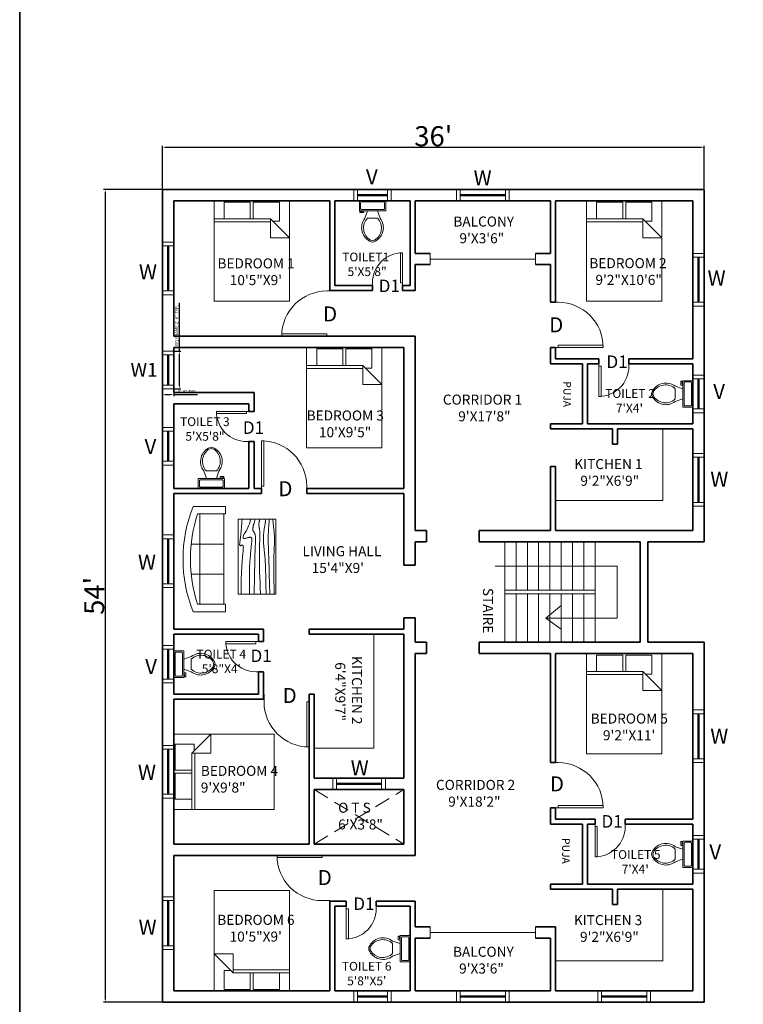
# Model space of a CAD drawing. Units: inches. Extents: x 2391 to 16591, y 7259 to 10239.
# Tile 17 of 27: x 2391 to 2968, y 8500 to 9285. Entities that reach past the tile are written whole.
import ezdxf

# ---------------------------------------------------------------- set-up
doc = ezdxf.new("R2010")
doc.units = ezdxf.units.IN
doc.linetypes.add('DASHED', pattern=[19.05, 12.7, -6.35])
for name, color, linetype, lineweight in [('A-ANNO-DIMS', 4, 'Continuous', 18), ('A-ANNO-IDEN', 2, 'Continuous', 18), ('A-ANNO-SYMB', 3, 'Continuous', 18), ('A-ANNO-TTLB', 7, 'Continuous', 35), ('A-AREA-IDEN', 7, 'Continuous', 18), ('A-DOOR', 3, 'Continuous', 18), ('A-FLOR-CASE', 6, 'Continuous', 18), ('A-FLOR-FIXT', 9, 'Continuous', 18), ('A-FLOR-HRAL', 8, 'Continuous', 18), ('A-FLOR-OPEN', 4, 'DASHED', 13), ('A-FLOR-STRS', 7, 'Continuous', 18), ('A-FURN', 8, 'Continuous', 18), ('A-GLAZ', 4, 'Continuous', 18), ('A-WALL', 7, 'Continuous', 35)]:
    doc.layers.add(name, color=color, linetype=linetype, lineweight=lineweight)
doc.styles.get("Standard").update_dxf_attribs({"font": 'arial.ttf'})
doc.dimstyles.new('ISO-25', dxfattribs={"dimtxt": 2.5, "dimasz": 2.5, "dimexe": 1.25, "dimexo": 0.625, "dimtad": 1, "dimdec": 0, "dimlunit": 3, "dimtxsty": 'Standard', "dimcen": 2.5, "dimadec": 0, "dimazin": 0, "dimtfac": 1, "dimtdec": 0, "dimtmove": 0, "dimatfit": 3, "dimfxl": 1, "dimarcsym": 0})

# ---------------------------------------------------------------- blocks, each defined once
blk = doc.blocks.new('Bed - Queen')
for p, q in [((0, -80.00003), (0, 0)), ((0, 0), (59.99999, 0)), ((59.99999, 0), (59.99999, -80.00003)), ((7.99999, -1.2), (28.79998, -1.2)), ((7.99999, -14.4), (7.99999, -1.2)), ((28.79998, -1.2), (28.79998, -14.4)), ((31.19999, -1.2), (51.99999, -1.2)), ((31.19999, -14.4), (31.19999, -1.2)), ((51.99999, -1.2), (51.99999, -16.4)), ((0, -14.4), (44.8, -14.4)), ((59.99999, -29.6), (44.8, -14.4)), ((44.8, -14.4), (44.8, -29.6)), ((44.8, -16.8), (0, -16.8)), ((51.99999, -16.4), (46.79936, -16.4)), ((44.8, -29.6), (59.99999, -29.6)), ((59.99999, -80.00003), (0, -80.00003))]:
    blk.add_line(p, q)
blk = doc.blocks.new('Toilet - top')
for p, q in [((9.5, -6), (9.5, -2)), ((-10, -8.5), (-8, -8.5)), ((-10, -9.5), (-10, -8.5)), ((-7, -9.5), (-10, -9.5)), ((-8, -8.5), (-8, -8)), ((-7, -8), (-7, -9.5)), ((-4, -8), (-6, -14)), ((4, -14), (-4, -14)), ((4, -8), (6, -14))]:
    blk.add_line(p, q)
blk.add_lwpolyline([(10.5, -8), (10.5, 0), (-10.5, 0), (-10.5, -8)], close=True)
for points in [[(-9.5, -2), (-9.5, -6)], [(8.5, -1), (-8.5, -1)], [(-8.5, -7), (8.5, -7)]]:
    blk.add_lwpolyline(points)
for centre, radius, start, end in [((-8.62, -1.88), 0.884, 81.8699, 188.1301), ((-8.62, -6.12), 0.884, 171.8699, 278.1301), ((8.62, -1.88), 0.884, 351.8699, 98.1301), ((8.62, -6.12), 0.884, 261.8699, 8.1301), ((3.52, -21.58), 12.17, 141.46911, 247.97143), ((4.2, -21.82), 11.33, 136.36773, 238.94682), ((-3.52, -21.58), 12.17, 292.02843, 38.53071), ((-4.2, -21.82), 11.33, 301.05301, 43.63209), ((0, -27.88), 4, 245.73182, 294.26817), ((0, -29), 4, 254.86053, 285.13947)]:
    blk.add_arc(centre, radius, start, end)
blk = doc.blocks.new('Sofa - Roundback 7 ft.')
for p, q in [((-12.00002, -32.4421), (-12.00003, -6.5971)), ((11.99997, -32.4421), (11.99998, -6.5971)), ((-36.000027, -34), (-36.000027, -11.4696)), ((-35.999844, -13.3819), (35.9998, -13.3819)), ((35.99998, -34), (35.99998, -11.4696)), ((-36.000027, -32.4421), (35.99998, -32.4421))]:
    blk.add_line(p, q)
for points in [[(-36.000027, -34), (-42.000027, -34), (-42.000027, -8)], [(41.99998, -8), (41.99998, -34), (35.99998, -34)]]:
    blk.add_lwpolyline(points)
for centre, radius, start, end in [((0, -114.25), 114.25, 68.43141, 111.5686), ((-0.00001, -127.1968), 121.1968, 72.72033, 107.2797)]:
    blk.add_arc(centre, radius, start, end)
blk = doc.blocks.new('Table - Rectangular Woodgrain 60 x 30 in.')
for p, q in [((0, 0), (0, -30)), ((60, 0), (0, 0)), ((60, -30), (60, 0)), ((0, -30), (60, -30))]:
    blk.add_line(p, q)
for points in [[(0, -2.4), (4.8155, -2.418), (9.0302, -2.4688), (12.709, -2.5477), (15.9167, -2.65), (18.7181, -2.7711), (21.1781, -2.9063), (23.3616, -3.0508), (25.3333, -3.2), (27.1477, -3.3495), (28.8172, -3.4958), (30.3437, -3.636), (31.7291, -3.7667), (32.9756, -3.8849), (34.0849, -3.9875), (35.059, -4.0714), (35.9, -4.1334), (36.6114, -4.1711), (37.2041, -4.1854), (37.6906, -4.1779), (38.0833, -4.15), (38.3948, -4.1034), (38.6375, -4.0396), (38.8239, -3.9602), (38.9666, -3.8667), (39.0764, -3.7608), (39.1573, -3.6448), (39.2116, -3.521), (39.2416, -3.3917), (39.2498, -3.2593), (39.2385, -3.1261), (39.21, -2.9944), (39.1666, -2.8667), (39.111, -2.7447), (39.0468, -2.6281), (38.978, -2.5163), (38.9083, -2.4083), (38.8418, -2.3035), (38.7823, -2.201), (38.7337, -2.1001), (38.7, -2), (38.6844, -1.9003), (38.6875, -1.8021), (38.7094, -1.707), (38.75, -1.6167), (38.8094, -1.5326), (38.8875, -1.4563), (38.9844, -1.3893), (39.1, -1.3333), (39.2351, -1.2896), (39.3937, -1.2583), (39.5804, -1.2396), (39.8, -1.2333), (40.057, -1.2396), (40.3562, -1.2583), (40.7023, -1.2896), (41.1, -1.3333), (41.5547, -1.3895), (42.0755, -1.4573), (42.6721, -1.5361), (43.3542, -1.625), (44.1316, -1.7233), (45.014, -1.8302), (46.0114, -1.9449), (47.1333, -2.0667), (48.3862, -2.1947), (49.7625, -2.3281), (51.2513, -2.4663), (52.8416, -2.6083), (54.5226, -2.7535), (56.2833, -2.9011), (58.1127, -3.0501), (60, -3.2)], [(0, -9.2), (6.5759, -9.0858), (11.9385, -9.0365), (16.2527, -9.0418), (19.6833, -9.0917), (22.3952, -9.1759), (24.5531, -9.2844), (26.322, -9.4069), (27.8666, -9.5333), (29.3241, -9.6553), (30.7203, -9.7719), (32.0532, -9.8837), (33.3208, -9.9917), (34.5213, -10.0965), (35.6526, -10.199), (36.7128, -10.2999), (37.7, -10.4), (38.6129, -10.4996), (39.4531, -10.5969), (40.223, -10.6895), (40.925, -10.775), (41.5613, -10.8512), (42.1344, -10.9156), (42.6465, -10.966), (43.1, -11), (43.4976, -11.0158), (43.8437, -11.0136), (44.143, -10.9942), (44.4, -10.9583), (44.6195, -10.9069), (44.8062, -10.8406), (44.9648, -10.7603), (45.1, -10.6667), (45.2155, -10.5598), (45.3114, -10.4365), (45.3871, -10.2929), (45.4416, -10.125), (45.4743, -9.929), (45.4844, -9.7011), (45.4709, -9.4371), (45.4333, -9.1333), (45.3716, -8.7883), (45.2896, -8.4104), (45.1919, -8.0107), (45.0833, -7.6), (44.9685, -7.1893), (44.8521, -6.7896), (44.7388, -6.4117), (44.6333, -6.0667), (44.54, -5.7628), (44.4614, -5.4979), (44.4001, -5.2675), (44.3583, -5.0667), (44.3384, -4.8909), (44.3427, -4.7354), (44.3736, -4.5956), (44.4333, -4.4667), (44.5236, -4.3453), (44.6427, -4.2333), (44.7884, -4.1339), (44.9583, -4.05), (45.1501, -3.9849), (45.3614, -3.9417), (45.59, -3.9234), (45.8333, -3.9333), (46.0915, -3.9749), (46.3734, -4.0531), (46.6906, -4.1736), (47.0542, -4.3417), (47.4756, -4.5629), (47.9661, -4.8427), (48.5372, -5.1866), (49.2, -5.6), (49.9676, -6.0844), (50.8594, -6.625), (51.8965, -7.2031), (53.1, -7.8), (54.491, -8.3969), (56.0906, -8.975), (57.9199, -9.5156), (60, -10)], [(0, -12.8), (5.1847, -12.9322), (9.6213, -13.0323), (13.3963, -13.1059), (16.5958, -13.1583), (19.3063, -13.1952), (21.614, -13.2219), (23.6054, -13.2439), (25.3666, -13.2667), (26.9728, -13.2947), (28.4531, -13.3281), (29.8256, -13.3663), (31.1083, -13.4083), (32.3191, -13.4535), (33.476, -13.501), (34.597, -13.5501), (35.7, -13.6), (36.7984, -13.6497), (37.8875, -13.6979), (38.9578, -13.743), (40, -13.7833), (41.0047, -13.8174), (41.9625, -13.8438), (42.864, -13.8607), (43.7, -13.8667), (44.4631, -13.8604), (45.1552, -13.8417), (45.7801, -13.8104), (46.3416, -13.7667), (46.8439, -13.7104), (47.2906, -13.6417), (47.6858, -13.5604), (48.0333, -13.4667), (48.3375, -13.3608), (48.6042, -13.2448), (48.8396, -13.121), (49.05, -12.9917), (49.2417, -12.8593), (49.4208, -12.7261), (49.5937, -12.5944), (49.7667, -12.4667), (49.9452, -12.3451), (50.1323, -12.2313), (50.3303, -12.1268), (50.5416, -12.0333), (50.7686, -11.9524), (51.0135, -11.8854), (51.2788, -11.8341), (51.5666, -11.8), (51.8785, -11.7843), (52.2116, -11.7865), (52.562, -11.8059), (52.926, -11.8417), (53.2998, -11.8931), (53.6795, -11.9594), (54.0614, -12.0397), (54.4416, -12.1333), (54.8223, -12.2401), (55.2293, -12.3625), (55.6942, -12.5037), (56.2489, -12.6667), (56.9251, -12.8547), (57.7545, -13.0708), (58.7689, -13.3182), (60, -13.6)], [(0, -18), (5.124, -17.7273), (9.6609, -17.5057), (13.6705, -17.3303), (17.2125, -17.1958), (20.3467, -17.0973), (23.1328, -17.0297), (25.6307, -16.9878), (27.9, -16.9667), (29.9928, -16.9617), (31.9302, -16.9703), (33.7254, -16.9907), (35.3917, -17.0208), (36.9423, -17.0588), (38.3906, -17.1026), (39.7499, -17.1503), (41.0333, -17.2), (42.2519, -17.2496), (43.4073, -17.2969), (44.4986, -17.3395), (45.525, -17.375), (46.4858, -17.4012), (47.3802, -17.4156), (48.2074, -17.416), (48.9667, -17.4), (49.6583, -17.3662), (50.2872, -17.3167), (50.8595, -17.2547), (51.3812, -17.1833), (51.8584, -17.1057), (52.2971, -17.025), (52.7034, -16.9443), (53.0833, -16.8667), (53.443, -16.7951), (53.789, -16.7313), (54.128, -16.6768), (54.4666, -16.6334), (54.8115, -16.6024), (55.1693, -16.5854), (55.5465, -16.5841), (55.95, -16.6), (56.3828, -16.6337), (56.8346, -16.6823), (57.2915, -16.7418), (57.7396, -16.8084), (58.165, -16.878), (58.5539, -16.9469), (58.8924, -17.0111), (59.1666, -17.0667), (59.3679, -17.1107), (59.5078, -17.1438), (59.6032, -17.1675), (59.6708, -17.1833), (59.7275, -17.193), (59.7901, -17.1979), (59.8753, -17.1998), (60, -17.2)], [(0, -22.4), (8.0098, -22.2501), (14.4094, -22.1011), (19.4168, -21.9535), (23.25, -21.8083), (26.1269, -21.6663), (28.2656, -21.5281), (29.884, -21.3947), (31.2, -21.2667), (32.3967, -21.1448), (33.5172, -21.0292), (34.5697, -20.9198), (35.5625, -20.8167), (36.5037, -20.7198), (37.4015, -20.6292), (38.2642, -20.5448), (39.1, -20.4667), (39.9164, -20.3951), (40.7187, -20.3313), (41.5117, -20.2768), (42.3, -20.2333), (43.0883, -20.2024), (43.8812, -20.1854), (44.6836, -20.1841), (45.5, -20.2), (46.3328, -20.234), (47.1747, -20.2844), (48.0163, -20.3488), (48.8479, -20.425), (49.66, -20.5106), (50.4429, -20.6031), (51.1872, -20.7004), (51.8833, -20.8), (52.5246, -20.8999), (53.1166, -20.9995), (53.6681, -21.0983), (54.1875, -21.1958), (54.6834, -21.2919), (55.1646, -21.3859), (55.6394, -21.4777), (56.1167, -21.5667), (56.6028, -21.6515), (57.0961, -21.7266), (57.5929, -21.7852), (58.0896, -21.8208), (58.5823, -21.8268), (59.0674, -21.7964), (59.5412, -21.723), (60, -21.6)], [(0, -25.2), (8.6355, -25.0504), (15.7026, -24.9031), (21.4049, -24.7606), (25.9458, -24.625), (29.529, -24.4988), (32.3578, -24.3844), (34.6359, -24.284), (36.5667, -24.2), (38.3213, -24.1341), (39.9417, -24.0854), (41.437, -24.0523), (42.8167, -24.0333), (44.0901, -24.0268), (45.2667, -24.0313), (46.3557, -24.0451), (47.3667, -24.0667), (48.309, -24.0947), (49.1928, -24.1287), (50.0284, -24.168), (50.826, -24.2125), (51.5959, -24.2617), (52.3483, -24.3151), (53.0935, -24.3725), (53.8417, -24.4334), (54.6009, -24.497), (55.3699, -24.561), (56.1454, -24.6226), (56.9239, -24.6792), (57.7021, -24.7279), (58.4764, -24.7662), (59.2435, -24.7911), (60, -24.8)], [(0, -28.8), (5.6867, -28.6681), (10.45, -28.5698), (14.407, -28.5012), (17.675, -28.4584), (20.3711, -28.4374), (22.6125, -28.4344), (24.5164, -28.4455), (26.2, -28.4667), (27.762, -28.4947), (29.2276, -28.5281), (30.6033, -28.5663), (31.8958, -28.6084), (33.1118, -28.6535), (34.2578, -28.7011), (35.3405, -28.7501), (36.3666, -28.8), (37.3443, -28.8497), (38.288, -28.8974), (39.2137, -28.9412), (40.1375, -28.9792), (41.0753, -29.0093), (42.0432, -29.0297), (43.0572, -29.0384), (44.1333, -29.0333), (45.2936, -29.0114), (46.5843, -28.9641), (48.0579, -28.8816), (49.7666, -28.7542), (51.7629, -28.5721), (54.0989, -28.3255), (56.8272, -28.0048), (60, -27.6)]]:
    blk.add_lwpolyline(points)
blk = doc.blocks.new('*U7')
for p, q in [((0, 0), (0, -6)), ((36, 0), (36, -6))]:
    blk.add_line(p, q)
blk.add_lwpolyline([(0, 0), (0, 36), (1.75, 36), (1.75, 0)], close=True)
blk.add_arc((0, 0), 36, 0, 90)
blk = doc.blocks.new('*U6')
for p, q in [((-36, 0), (-36, 6)), ((0, 0), (0, 6))]:
    blk.add_line(p, q)
blk.add_lwpolyline([(0, 0), (0, -36), (-1.75, -36), (-1.75, 0)], close=True)
blk.add_arc((0, 0), 36, 180, 270)
blk = doc.blocks.new('*U8')
for p, q in [((-24, 0), (-24, -6)), ((0, 0), (0, -6))]:
    blk.add_line(p, q)
blk.add_lwpolyline([(0, 0), (0, 24), (-1.75, 24), (-1.75, 0)], close=True)
blk.add_arc((0, 0), 24, 90, 180)
blk = doc.blocks.new('*U9')
for p, q in [((0, 0), (0, 6)), ((24, 0), (24, 6))]:
    blk.add_line(p, q)
blk.add_lwpolyline([(0, 0), (0, -24), (1.75, -24), (1.75, 0)], close=True)
blk.add_arc((0, 0), 24, 270, 0)
blk = doc.blocks.new('*U10')
for p, q in [((0, 0), (0, -6)), ((-36, 0), (-36, -6))]:
    blk.add_line(p, q)
blk.add_lwpolyline([(0, 0), (0, 36), (-1.75, 36), (-1.75, 0)], close=True)
blk.add_arc((0, 0), 36, 90, 180)
blk = doc.blocks.new('*U11')
for p, q in [((-36, 0), (-36, 6)), ((0, 0), (0, 6))]:
    blk.add_line(p, q)
blk.add_lwpolyline([(0, 0), (0, -36), (-1.75, -36), (-1.75, 0)], close=True)
blk.add_arc((0, 0), 36, 180, 270)
blk = doc.blocks.new('*U12')
for p, q in [((0, 0), (0, -6)), ((-36, 0), (-36, -6))]:
    blk.add_line(p, q)
blk.add_lwpolyline([(0, 0), (0, 36), (-1.75, 36), (-1.75, 0)], close=True)
blk.add_arc((0, 0), 36, 90, 180)
blk = doc.blocks.new('*U13')
for p, q in [((0, 0), (0, 6)), ((36, 0), (36, 6))]:
    blk.add_line(p, q)
blk.add_lwpolyline([(0, 0), (0, -36), (1.75, -36), (1.75, 0)], close=True)
blk.add_arc((0, 0), 36, 270, 0)
blk = doc.blocks.new('*D14')
at = {"layer": 'A-ANNO-DIMS', "color": 0, "lineweight": -2, "transparency": 16777216}
for p, q in [((2505.16, 9150.16), (2505.16, 9184.36)), ((2937.16, 9150.16), (2937.16, 9184.36)), ((2507.66, 9183.11), (2934.66, 9183.11))]:
    blk.add_line(p, q, dxfattribs=at)
at = {"layer": 'A-ANNO-DIMS', "color": 0, "transparency": 16777216}
for points in [[(2507.66, 9183.53), (2507.66, 9182.7), (2505.16, 9183.11)], [(2934.66, 9183.53), (2934.66, 9182.7), (2937.16, 9183.11)]]:
    blk.add_solid(points, dxfattribs=at)
at = {"layer": 'Defpoints', "color": 0, "transparency": 16777216}
for p in [(2937.16, 9183.11), (2505.16, 9149.53), (2937.16, 9149.53)]:
    blk.add_point(p, dxfattribs=at)
at = {"layer": 'A-ANNO-DIMS', "color": 0, "transparency": 16777216, "insert": (2721.16, 9191.91), "char_height": 2.5, "attachment_point": 5}
blk.add_mtext("{\\H6.4x;36'}", dxfattribs=at)
blk = doc.blocks.new('*D15')
at = {"layer": 'A-ANNO-DIMS', "color": 0, "lineweight": -2, "transparency": 16777216}
for p, q in [((2504.54, 9149.53), (2458.23, 9149.53)), ((2459.48, 9147.03), (2459.48, 8504.03)), ((2504.54, 8501.53), (2458.23, 8501.53))]:
    blk.add_line(p, q, dxfattribs=at)
at = {"layer": 'A-ANNO-DIMS', "color": 0, "transparency": 16777216}
for points in [[(2459.06, 9147.03), (2459.89, 9147.03), (2459.48, 9149.53)], [(2459.06, 8504.03), (2459.89, 8504.03), (2459.48, 8501.53)]]:
    blk.add_solid(points, dxfattribs=at)
at = {"layer": 'Defpoints', "color": 0, "transparency": 16777216}
for p in [(2505.16, 9149.53), (2459.48, 8501.53), (2505.16, 8501.53)]:
    blk.add_point(p, dxfattribs=at)
at = {"layer": 'A-ANNO-DIMS', "color": 0, "transparency": 16777216, "insert": (2450.71, 8825.53), "char_height": 2.5, "attachment_point": 5, "rotation": 90}
blk.add_mtext("{\\H6.4x;54'}", dxfattribs=at)
blk = doc.blocks.new('WINDOW-36-PLAN')
for p, q in [((9, 42), (0, 42)), ((9, 39), (0, 39)), ((4, 39), (4, 3)), ((4.5, 39), (4.5, 3)), ((5, 39), (5, 3)), ((9, 3), (0, 3)), ((9, 0), (0, 0))]:
    blk.add_line(p, q)
blk = doc.blocks.new('VENT-24-PLAN')
for p, q in [((9, 30), (0, 30)), ((9, 27), (0, 27)), ((4, 27), (4, 3)), ((4.5, 27), (4.5, 3)), ((5, 27), (5, 3)), ((9, 3), (0, 3)), ((9, 0), (0, 0))]:
    blk.add_line(p, q)
blk = doc.blocks.new('WINDOW-24-PLAN')
for p, q in [((9, 30), (0, 30)), ((9, 27), (0, 27)), ((4, 27), (4, 3)), ((4.5, 27), (4.5, 3)), ((5, 27), (5, 3)), ((9, 3), (0, 3)), ((9, 0), (0, 0))]:
    blk.add_line(p, q)
blk = doc.blocks.new('STAIR-RETURN-FLIGHT')
for p, q in [((0, 80), (0, 0)), ((9, 80), (9, 41.5)), ((18, 80), (18, 41.5)), ((27, 80), (27, 41.5)), ((36, 80), (36, 41.5)), ((45, 80), (45, 41.5)), ((54, 80), (54, 41.5)), ((63, 80), (63, 41.5)), ((72, 80), (72, 0)), ((72, 41.5), (0, 41.5)), ((72, 38.5), (0, 38.5)), ((9, 38.5), (9, 0)), ((18, 38.5), (18, 0)), ((27, 38.5), (27, 0)), ((36, 38.5), (36, 0)), ((45, 38.5), (45, 0)), ((54, 38.5), (54, 0)), ((63, 38.5), (63, 0))]:
    blk.add_line(p, q)
blk = doc.blocks.new('STAIR-DIRECTION-ARROW')
for p, q in [((0, 50.31), (97.37, 50.31)), ((97.37, 50.31), (97.37, 8.81)), ((40.34, 8.81), (52.74, 18.89)), ((97.37, 8.81), (40.34, 8.81)), ((40.34, 8.81), (52.74, 0))]:
    blk.add_line(p, q)
blk = doc.blocks.new('COUNTER-L-RETURN')
for q in [(47.5, 91), (0, 0)]:
    blk.add_line((47.5, 0), q)
blk = doc.blocks.new('COUNTER-L-KITCHEN')
for p, q in [((85.5, 57), (85.5, 0)), ((85.5, 0), (0, 0))]:
    blk.add_line(p, q)
blk = doc.blocks.new('*D41')
at = {"layer": 'A-ANNO-DIMS', "color": 0, "lineweight": -2, "transparency": 16777216}
for p, q in [((2518.66, 9020.53), (2518.66, 9059.02)), ((2514.79, 9020.53), (2519.91, 9020.53)), ((2518.66, 8993.03), (2518.66, 9018.03)), ((2514.79, 8990.53), (2519.91, 8990.53))]:
    blk.add_line(p, q, dxfattribs=at)
at = {"layer": 'A-ANNO-DIMS', "color": 0, "transparency": 16777216}
for points in [[(2518.24, 9018.03), (2519.08, 9018.03), (2518.66, 9020.53)], [(2518.24, 8993.03), (2519.08, 8993.03), (2518.66, 8990.53)]]:
    blk.add_solid(points, dxfattribs=at)
at = {"layer": 'Defpoints', "color": 0, "transparency": 16777216}
for p in [(2514.16, 9020.53), (2518.66, 9020.53), (2514.16, 8990.53)]:
    blk.add_point(p, dxfattribs=at)
at = {"layer": 'A-ANNO-DIMS', "color": 0, "transparency": 16777216, "insert": (2516.76, 9041.03), "char_height": 2.5, "attachment_point": 5, "rotation": 90}
blk.add_mtext('W1 FRAME 2\'-6" TYP.', dxfattribs=at)
blk = doc.blocks.new('*D42')
at = {"layer": 'A-ANNO-DIMS', "color": 0, "lineweight": -2, "transparency": 16777216}
for p, q in [((2505.16, 8989.91), (2505.16, 8984.78)), ((2514.16, 8989.91), (2514.16, 8984.78)), ((2507.66, 8986.03), (2511.66, 8986.03)), ((2514.16, 8986.03), (2533.15, 8986.03))]:
    blk.add_line(p, q, dxfattribs=at)
at = {"layer": 'A-ANNO-DIMS', "color": 0, "transparency": 16777216}
for points in [[(2507.66, 8986.45), (2507.66, 8985.61), (2505.16, 8986.03)], [(2511.66, 8986.45), (2511.66, 8985.61), (2514.16, 8986.03)]]:
    blk.add_solid(points, dxfattribs=at)
at = {"layer": 'Defpoints', "color": 0, "transparency": 16777216}
for p in [(2505.16, 8990.53), (2514.16, 8990.53), (2514.16, 8986.03)]:
    blk.add_point(p, dxfattribs=at)
at = {"layer": 'A-ANNO-DIMS', "color": 0, "transparency": 16777216, "insert": (2524.9, 8987.93), "char_height": 2.5, "attachment_point": 5}
blk.add_mtext('0\'-9" TYP.', dxfattribs=at)

msp = doc.modelspace()

# ---------------------------------------------------------------- linework, layer by layer
at = {"layer": 'A-ANNO-TTLB'}
msp.add_lwpolyline([(2391.28, 10239.38), (4154.2, 10239.38), (4154.2, 7258.54), (2391.28, 7258.54)], close=True, dxfattribs=at)
at = {"layer": 'A-DOOR'}
msp.add_line((2638.51, 8618.53), (2638.51, 8618.53), dxfattribs=at)
at = {"layer": 'A-FLOR-HRAL'}
for p, q in [((2718.66, 9089.53), (2718.66, 9098.53)), ((2802.66, 9089.53), (2802.66, 9098.53)), ((2718.66, 9094.03), (2802.66, 9094.03)), ((2718.66, 8552.53), (2718.66, 8561.53)), ((2718.66, 8557.03), (2802.66, 8557.03)), ((2802.66, 8552.53), (2802.66, 8561.53))]:
    msp.add_line(p, q, dxfattribs=at)
at = {"layer": 'A-FLOR-OPEN'}
for p, q in [((2626.16, 8627.53), (2697.66, 8671.03)), ((2626.16, 8671.03), (2697.66, 8627.53))]:
    msp.add_line(p, q, dxfattribs=at)
at = {"layer": 'A-WALL'}
for p, q in [((2505.16, 9149.53), (2937.16, 9149.53)), ((2505.16, 8501.53), (2505.16, 9149.53)), ((2937.16, 9149.53), (2937.16, 8868.53)), ((2514.16, 9140.53), (2638.66, 9140.53)), ((2514.16, 9032.53), (2514.16, 9140.53)), ((2638.66, 9069.03), (2638.66, 9140.53)), ((2642.66, 9073.03), (2642.66, 9140.53)), ((2642.66, 9140.53), (2702.66, 9140.53)), ((2702.66, 9073.03), (2702.66, 9140.53)), ((2706.66, 9098.53), (2706.66, 9140.53)), ((2706.66, 9140.53), (2814.66, 9140.53)), ((2814.66, 9098.53), (2814.66, 9140.53)), ((2818.66, 9059.53), (2818.66, 9140.53)), ((2818.66, 9140.53), (2928.16, 9140.53)), ((2928.16, 9140.53), (2928.16, 9014.53)), ((2706.66, 9098.53), (2718.66, 9098.53)), ((2802.66, 9098.53), (2814.66, 9098.53)), ((2706.66, 9089.53), (2718.66, 9089.53)), ((2706.66, 9069.03), (2706.66, 9089.53)), ((2802.66, 9089.53), (2814.66, 9089.53)), ((2814.66, 9059.53), (2814.66, 9089.53)), ((2638.66, 9069.03), (2672.66, 9069.03)), ((2642.66, 9073.03), (2672.66, 9073.03)), ((2672.66, 9069.03), (2672.66, 9073.03)), ((2696.66, 9069.03), (2696.66, 9073.03)), ((2696.66, 9073.03), (2702.66, 9073.03)), ((2696.66, 9069.03), (2706.66, 9069.03)), ((2814.66, 9059.53), (2818.66, 9059.53)), ((2514.16, 9032.53), (2706.66, 9032.53)), ((2706.66, 8877.53), (2706.66, 9032.53)), ((2514.16, 9023.53), (2697.66, 9023.53)), ((2514.16, 8987.53), (2514.16, 9023.53)), ((2697.66, 8911.03), (2697.66, 9023.53)), ((2814.66, 9010.53), (2814.66, 9023.53)), ((2814.66, 9023.53), (2818.66, 9023.53)), ((2818.66, 9014.53), (2818.66, 9023.53)), ((2818.66, 9014.53), (2853.16, 9014.53)), ((2853.16, 9014.53), (2853.16, 9010.53)), ((2877.16, 9014.53), (2877.16, 9010.53)), ((2877.16, 9014.53), (2928.16, 9014.53)), ((2814.66, 9010.53), (2840.16, 9010.53)), ((2840.16, 9010.53), (2840.16, 8962.53)), ((2844.16, 9010.53), (2844.16, 8962.53)), ((2844.16, 9010.53), (2853.16, 9010.53)), ((2877.16, 9010.53), (2928.16, 9010.53)), ((2928.16, 9010.53), (2928.16, 8962.53)), ((2514.16, 8987.53), (2578.16, 8987.53)), ((2578.16, 8972.53), (2578.16, 8987.53)), ((2514.16, 8978.53), (2574.16, 8978.53)), ((2514.16, 8911.03), (2514.16, 8978.53)), ((2574.16, 8972.53), (2574.16, 8978.53)), ((2574.16, 8972.53), (2578.16, 8972.53)), ((2814.66, 8962.53), (2840.16, 8962.53)), ((2814.66, 8958.53), (2814.66, 8962.53)), ((2814.66, 8958.53), (2864.16, 8958.53)), ((2844.16, 8962.53), (2928.16, 8962.53)), ((2864.16, 8958.53), (2864.16, 8946.53)), ((2868.16, 8958.53), (2868.16, 8946.53)), ((2868.16, 8958.53), (2928.16, 8958.53)), ((2928.16, 8958.53), (2928.16, 8877.53)), ((2574.16, 8911.03), (2574.16, 8948.53)), ((2574.16, 8948.53), (2578.16, 8948.53)), ((2578.16, 8911.03), (2578.16, 8948.53)), ((2864.16, 8946.53), (2868.16, 8946.53)), ((2814.66, 8877.53), (2814.66, 8928.53)), ((2814.66, 8928.53), (2818.66, 8928.53)), ((2818.66, 8877.53), (2818.66, 8928.53)), ((2514.16, 8911.03), (2574.16, 8911.03)), ((2578.16, 8911.03), (2584.16, 8911.03)), ((2584.16, 8907.03), (2584.16, 8911.03)), ((2620.16, 8907.03), (2620.16, 8911.03)), ((2620.16, 8911.03), (2697.66, 8911.03)), ((2514.16, 8907.03), (2584.16, 8907.03)), ((2514.16, 8799.03), (2514.16, 8907.03)), ((2620.16, 8907.03), (2697.66, 8907.03)), ((2697.66, 8850.03), (2697.66, 8907.03)), ((2706.66, 8877.53), (2715.66, 8877.53)), ((2715.66, 8868.53), (2715.66, 8877.53)), ((2757.66, 8868.53), (2757.66, 8877.53)), ((2757.66, 8877.53), (2814.66, 8877.53)), ((2818.66, 8877.53), (2928.16, 8877.53)), ((2706.66, 8868.53), (2715.66, 8868.53)), ((2706.66, 8850.03), (2706.66, 8868.53)), ((2757.66, 8868.53), (2886.16, 8868.53)), ((2886.16, 8868.53), (2886.16, 8788.53)), ((2892.16, 8868.53), (2892.16, 8788.53)), ((2892.16, 8868.53), (2937.16, 8868.53)), ((2697.66, 8850.03), (2706.66, 8850.03)), ((2697.66, 8799.03), (2697.66, 8808.03)), ((2697.66, 8808.03), (2706.66, 8808.03)), ((2706.66, 8788.53), (2706.66, 8808.03)), ((2514.16, 8799.03), (2585.66, 8799.03)), ((2514.16, 8795.03), (2581.66, 8795.03)), ((2514.16, 8747.03), (2514.16, 8795.03)), ((2581.66, 8789.03), (2581.66, 8795.03)), ((2585.66, 8789.03), (2585.66, 8799.03)), ((2622.16, 8795.03), (2622.16, 8799.03)), ((2622.16, 8799.03), (2697.66, 8799.03)), ((2622.16, 8795.03), (2697.66, 8795.03)), ((2697.66, 8680.03), (2697.66, 8795.03)), ((2581.66, 8789.03), (2585.66, 8789.03)), ((2715.66, 8788.53), (2706.66, 8788.53)), ((2715.66, 8779.53), (2715.66, 8788.53)), ((2886.16, 8788.53), (2757.66, 8788.53)), ((2757.66, 8779.53), (2757.66, 8788.53)), ((2937.16, 8788.53), (2892.16, 8788.53)), ((2937.16, 8788.53), (2937.16, 8501.53)), ((2715.66, 8779.53), (2706.66, 8779.53)), ((2706.66, 8618.53), (2706.66, 8779.53)), ((2814.66, 8779.53), (2757.66, 8779.53)), ((2814.66, 8692.53), (2814.66, 8779.53)), ((2928.16, 8779.53), (2818.66, 8779.53)), ((2818.66, 8692.53), (2818.66, 8779.53)), ((2928.16, 8779.53), (2928.16, 8647.53)), ((2581.66, 8747.03), (2581.66, 8765.03)), ((2581.66, 8765.03), (2585.66, 8765.03)), ((2585.66, 8743.03), (2585.66, 8765.03)), ((2514.16, 8747.03), (2581.66, 8747.03)), ((2622.16, 8627.53), (2622.16, 8747.03)), ((2622.16, 8747.03), (2626.16, 8747.03)), ((2626.16, 8680.03), (2626.16, 8747.03)), ((2514.16, 8743.03), (2585.66, 8743.03)), ((2514.16, 8627.53), (2514.16, 8743.03)), ((2818.66, 8692.53), (2814.66, 8692.53)), ((2697.66, 8680.03), (2626.16, 8680.03)), ((2626.16, 8627.53), (2626.16, 8671.03)), ((2697.66, 8671.03), (2626.16, 8671.03)), ((2697.66, 8627.53), (2697.66, 8671.03)), ((2814.66, 8643.53), (2814.66, 8656.53)), ((2818.66, 8656.53), (2814.66, 8656.53)), ((2818.66, 8647.53), (2818.66, 8656.53)), ((2840.16, 8643.53), (2814.66, 8643.53)), ((2850.16, 8647.53), (2818.66, 8647.53)), ((2840.16, 8643.53), (2840.16, 8595.53)), ((2844.16, 8643.53), (2844.16, 8595.53)), ((2850.16, 8643.53), (2844.16, 8643.53)), ((2850.16, 8647.53), (2850.16, 8643.53)), ((2928.16, 8647.53), (2874.16, 8647.53)), ((2874.16, 8647.53), (2874.16, 8643.53)), ((2928.16, 8643.53), (2874.16, 8643.53)), ((2928.16, 8643.53), (2928.16, 8595.53)), ((2622.16, 8627.53), (2514.16, 8627.53)), ((2697.66, 8627.53), (2626.16, 8627.53)), ((2514.16, 8510.53), (2514.16, 8618.53)), ((2642.66, 8618.53), (2514.16, 8618.53)), ((2706.66, 8618.53), (2642.66, 8618.53)), ((2814.66, 8591.53), (2814.66, 8595.53)), ((2840.16, 8595.53), (2814.66, 8595.53)), ((2928.16, 8595.53), (2844.16, 8595.53)), ((2864.16, 8591.53), (2814.66, 8591.53)), ((2864.16, 8591.53), (2864.16, 8579.53)), ((2928.16, 8591.53), (2868.16, 8591.53)), ((2868.16, 8591.53), (2868.16, 8579.53)), ((2928.16, 8591.53), (2928.16, 8510.53)), ((2638.66, 8510.53), (2638.66, 8582.03)), ((2651.66, 8582.03), (2638.66, 8582.03)), ((2651.66, 8578.03), (2651.66, 8582.03)), ((2706.66, 8582.03), (2675.66, 8582.03)), ((2675.66, 8578.03), (2675.66, 8582.03)), ((2706.66, 8561.53), (2706.66, 8582.03)), ((2642.66, 8510.53), (2642.66, 8578.03)), ((2651.66, 8578.03), (2642.66, 8578.03)), ((2702.66, 8578.03), (2675.66, 8578.03)), ((2702.66, 8510.53), (2702.66, 8578.03)), ((2868.16, 8579.53), (2864.16, 8579.53)), ((2718.66, 8561.53), (2706.66, 8561.53)), ((2818.66, 8561.53), (2802.66, 8561.53)), ((2818.66, 8510.53), (2818.66, 8561.53)), ((2706.66, 8510.53), (2706.66, 8552.53)), ((2718.66, 8552.53), (2706.66, 8552.53)), ((2814.66, 8552.53), (2802.66, 8552.53)), ((2814.66, 8510.53), (2814.66, 8552.53)), ((2638.66, 8510.53), (2514.16, 8510.53)), ((2702.66, 8510.53), (2642.66, 8510.53)), ((2814.66, 8510.53), (2706.66, 8510.53)), ((2928.16, 8510.53), (2818.66, 8510.53)), ((2937.16, 8501.53), (2505.16, 8501.53))]:
    msp.add_line(p, q, dxfattribs=at)

# ---------------------------------------------------------------- block references
at = {"layer": 'A-ANNO-SYMB'}
msp.add_blockref('STAIR-DIRECTION-ARROW', (2770.42, 8798.98), dxfattribs=at)
at = {"layer": 'A-DOOR'}
for name, p in [('*U8', (2696.66, 9075.03)), ('*U9', (2853.16, 9008.53)), ('*U7', (2584.16, 8913.03)), ('*U6', (2622.16, 8741.03)), ('*U9', (2850.16, 8641.53)), ('*U9', (2651.66, 8576.03))]:
    msp.add_blockref(name, p, dxfattribs=at)
at = {"layer": 'A-DOOR', "rotation": 270}
for name, p in [('*U11', (2636.26, 9032.53)), ('*U12', (2820.66, 9023.53)), ('*U9', (2572.16, 8972.53)), ('*U9', (2579.66, 8789.03)), ('*U10', (2820.66, 8656.53)), ('*U13', (2632.51, 8618.53))]:
    msp.add_blockref(name, p, dxfattribs=at)
at = {"layer": 'A-FLOR-CASE'}
for name, p in [('COUNTER-L-KITCHEN', (2818.66, 8901.53)), ('COUNTER-L-RETURN', (2626.16, 8704.03)), ('COUNTER-L-KITCHEN', (2818.66, 8534.53))]:
    msp.add_blockref(name, p, dxfattribs=at)
at = {"layer": 'A-FLOR-FIXT'}
msp.add_blockref('Toilet - top', (2672.66, 9140.53), dxfattribs=at)
for p, rotation in [((2928.16, 8986.53), 270), ((2544.16, 8911.03), 180), ((2514.16, 8771.03), 89.99999999999999), ((2928.16, 8619.53), 270), ((2702.66, 8544.28), 270)]:
    msp.add_blockref('Toilet - top', p, dxfattribs=dict(at, rotation=rotation))
at = {"layer": 'A-FLOR-STRS'}
msp.add_blockref('STAIR-RETURN-FLIGHT', (2778.16, 8788.53), dxfattribs=at)
at = {"layer": 'A-FURN'}
for p in [(2546.41, 9140.53), (2843.41, 9140.53), (2620.13, 9023.53), (2843.41, 8779.53)]:
    msp.add_blockref('Bed - Queen', p, dxfattribs=at)
for name, p, rotation in [('Sofa - Roundback 7 ft.', (2521.55, 8854.81), 90), ('Table - Rectangular Woodgrain 60 x 30 in.', (2565.46, 8826.76), 90), ('Bed - Queen', (2514.16, 8655.28), 90), ('Bed - Queen', (2606.41, 8510.53), 180)]:
    msp.add_blockref(name, p, dxfattribs=dict(at, rotation=rotation))
at = {"layer": 'A-GLAZ'}
for name, p, rotation in [('VENT-24-PLAN', (2657.66, 9149.53), 269.9999999999936), ('WINDOW-36-PLAN', (2739.66, 9149.53), 270), ('WINDOW-36-PLAN', (2640.91, 8680.03), 269.9999999999998), ('VENT-24-PLAN', (2657.66, 8510.53), 270.0000000000005), ('WINDOW-36-PLAN', (2739.66, 8510.53), 269.9999999999995), ('WINDOW-36-PLAN', (2852.41, 8510.53), 270)]:
    msp.add_blockref(name, p, dxfattribs=dict(at, rotation=rotation))
for name, p in [('WINDOW-36-PLAN', (2505.16, 9065.53)), ('WINDOW-36-PLAN', (2928.16, 9056.53)), ('WINDOW-24-PLAN', (2505.16, 8990.53)), ('VENT-24-PLAN', (2928.16, 8971.53)), ('VENT-24-PLAN', (2505.16, 8929.78)), ('WINDOW-36-PLAN', (2928.16, 8897.03)), ('WINDOW-36-PLAN', (2505.16, 8832.03)), ('VENT-24-PLAN', (2505.16, 8756.03)), ('WINDOW-36-PLAN', (2928.16, 8692.53)), ('WINDOW-36-PLAN', (2505.16, 8664.28)), ('VENT-24-PLAN', (2928.16, 8604.53)), ('WINDOW-36-PLAN', (2505.16, 8543.53))]:
    msp.add_blockref(name, p, dxfattribs=at)

# ---------------------------------------------------------------- texts
at = {"layer": 'A-ANNO-IDEN', "attachment_point": 1}
for s, width, insert, char_height in [('V', 33.2285, (2667.43, 9165.53), 12), ('W', 41.0391, (2753.28, 9164.73), 12), ('W', 25.6098, (2486.38, 9089.72), 12), ('W', 63.2637, (2939.89, 9084.88), 12), ('D1', 88.0557, (2677.57, 9077.64), 10), ('D', 711.4851, (2633.21, 9056.24), 12), ('D', 1570.4564, (2813.57, 9047.55), 12), ('D1', 69.9915, (2859.21, 9017.11), 10), ('W1', 26.8712, (2479.71, 9011.17), 11), ('V', 60.3219, (2944.36, 8994.49), 12), ('D1', 74.2476, (2569.24, 8964.63), 10), ('V', 17.0712, (2490.85, 8950.59), 12), ('W', 105.2929, (2942.06, 8924.44), 12), ('D ', 382.5297, (2597.57, 8916.92), 12), ('W', 40.7205, (2485.59, 8858.35), 12), ('D1', 102.8831, (2575.36, 8782.67), 10), ('V', 16.5796, (2491.34, 8775.11), 12), ('D', 433.7706, (2600.98, 8752.05), 12), ('W', 123.7268, (2942.02, 8719.74), 12), ('W', 28.3648, (2485.57, 8690.78), 12), ('W', 47.6363, (2655.25, 8694.41), 12), ('D', 235.1744, (2814.11, 8681.59), 12), ('D1', 70.0055, (2855.27, 8650.73), 10), ('V', 48.5524, (2941.27, 8627.33), 12), ('D', 460.223, (2628.97, 8606.89), 12), ('D1', 90.0045, (2657.36, 8585.09), 10), ('W', 32.8374, (2486.09, 8567.27), 12)]:
    msp.add_mtext_dynamic_manual_height_columns(s, width=width, gutter_width=12.5, heights=[0], dxfattribs=dict(at, insert=insert, char_height=char_height))
at = {"layer": 'A-AREA-IDEN', "attachment_point": 1}
for s, width, insert, char_height in [('BALCONY\\P  9\'X3\'6"', 125.309, (2737.11, 9127.91), 8), ('TOILET1\\P  5\'X5\'8"', 175.2431, (2648.5, 9099.14), 7), ('BEDROOM 1\\P    10\'5"X9\'', 152.4027, (2549.01, 9094.55), 8), ('BEDROOM 2\\P  9\'2"X10\'6"', 186.7643, (2845.58, 9094.72), 8), ("{\\H0.875x;TOILET 2\\P    7'X4}'", 130.8261, (2858.24, 8990.3), 8), ('CORRIDOR 1\\P     9\'X17\'8"', 386.0733, (2728.79, 8985.94), 8), ('BEDROOM 3\\P    10\'X9\'5"', 134.4574, (2620.13, 8973.29), 8), ('TOILET 3\\P  5\'X5\'8"', 110.3725, (2519.16, 8967.85), 7), ('KITCHEN 1\\P  9\'2"X6\'9"', 260.4884, (2833.53, 8934.57), 8), ('LIVING HALL\\P   15\'4"X9\'', 316.1653, (2616.79, 8865.07), 8), ('TOILET 4\\P  5\'8"X4\'', 115.6049, (2532.24, 8782.53), 7), ('BEDROOM 5\\P    9\'2"X11\'', 234.3403, (2846.65, 8731.68), 8), ('BEDROOM 4\\P9\'X9\'8"', 337.9313, (2535.72, 8689.98), 8), ('CORRIDOR 2\\P    9\'X18\'2"  ', 260.1533, (2723.26, 8678.78), 8), ('O T S\\P6\'X3\'8"', 143.5906, (2645.27, 8660.58), 8), ("{\\H0.875x;TOILET 5\\P    7'X4}'", 130.8261, (2862.84, 8622.76), 8), ('BEDROOM 6\\P    10\'5"X9\'', 279.7405, (2548.89, 8571.2), 8), ('KITCHEN 3\\P  9\'2"X6\'9"', 205.0668, (2833.25, 8570.98), 8), ('BALCONY\\P  9\'X3\'6"', 151.3379, (2736.85, 8545.72), 8), ('TOILET 6\\P  5\'8"X5\'', 210.0226, (2648.22, 8533.7), 7)]:
    msp.add_mtext_dynamic_manual_height_columns(s, width=width, gutter_width=12.5, heights=[0], dxfattribs=dict(at, insert=insert, char_height=char_height))
at = {"layer": 'A-AREA-IDEN', "attachment_point": 1, "rotation": 270}
for s, width, insert, char_height in [('PUJA', 212.5876, (2830.92, 8996.5), 6), ('STAIRE', 212.5876, (2768.83, 8831.83), 8), ('KITCHEN 2\\P  6\'4"X9\'7"', 154.6668, (2664.27, 8777.49), 8), ('PUJA', 212.5876, (2829.9, 8632.37), 6)]:
    msp.add_mtext_dynamic_manual_height_columns(s, width=width, gutter_width=12.5, heights=[0], dxfattribs=dict(at, insert=insert, char_height=char_height))

# ---------------------------------------------------------------- dimensions: what is measured, and where the dimension line sits
at = {"layer": 'A-ANNO-DIMS'}
for base, p1, p2, text, override, picture, middle in [((2937.16, 9183.11), (2505.16, 9149.53), (2937.16, 9149.53), '{\\H6.4x;<>}', {"dimclrd": 0, "dimclre": 0, "dimclrt": 0}, '*D14', (2721.16, 9191.91)), ((2514.16, 8986.03), (2505.16, 8990.53), (2514.16, 8990.53), '<> TYP.', {"dimdec": 1, "dimlfac": 1, "dimrnd": 0, "dimzin": 1, "dimdsep": 46, "dimlunit": 4, "dimfrac": 2}, '*D42', (2524.9, 8987.93))]:
    dim = msp.add_linear_dim(base=base, p1=p1, p2=p2, text=text, dimstyle='ISO-25', override=override, dxfattribs=at)
    dim.commit()
    dim.dimension.update_dxf_attribs({"geometry": picture, "text_midpoint": middle})
for base, p1, p2, text, override, picture, middle in [((2459.48, 8501.53), (2505.16, 9149.53), (2505.16, 8501.53), '{\\H6.4x;<>}', {"dimclrd": 0, "dimclre": 0, "dimclrt": 0}, '*D15', (2450.71, 8825.53)), ((2518.66, 9020.53), (2514.16, 8990.53), (2514.16, 9020.53), 'W1 FRAME <> TYP.', {"dimdec": 1, "dimlfac": 1, "dimrnd": 0, "dimzin": 1, "dimdsep": 46, "dimlunit": 4, "dimfrac": 2}, '*D41', (2516.76, 9041.03))]:
    dim = msp.add_linear_dim(base=base, p1=p1, p2=p2, angle=90, text=text, dimstyle='ISO-25', override=override, dxfattribs=at)
    dim.commit()
    dim.dimension.update_dxf_attribs({"geometry": picture, "text_midpoint": middle})

doc.saveas('drawing.dxf')
